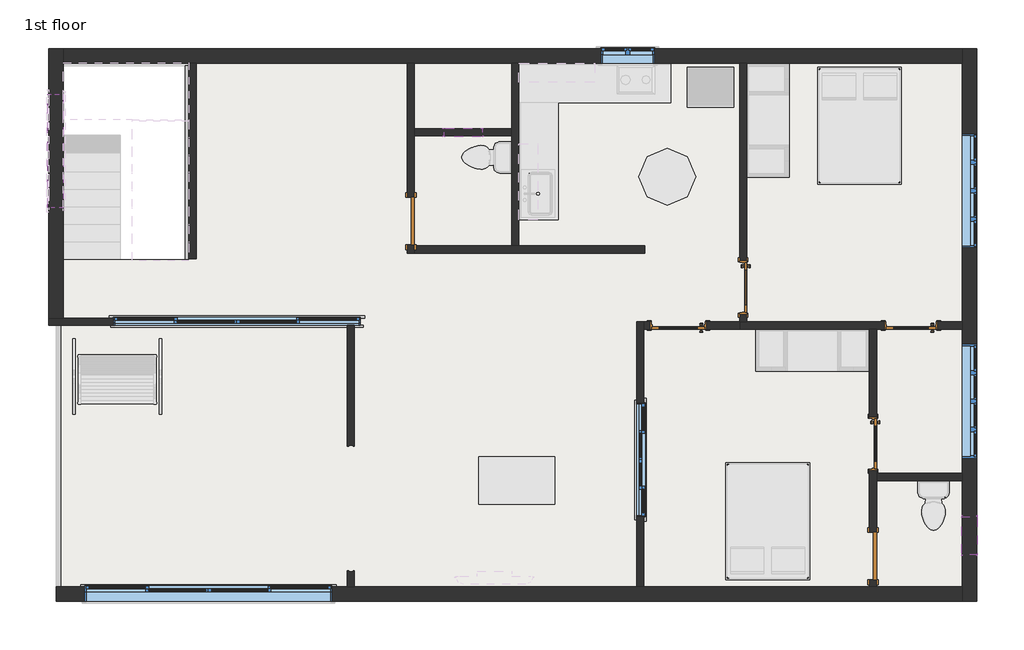
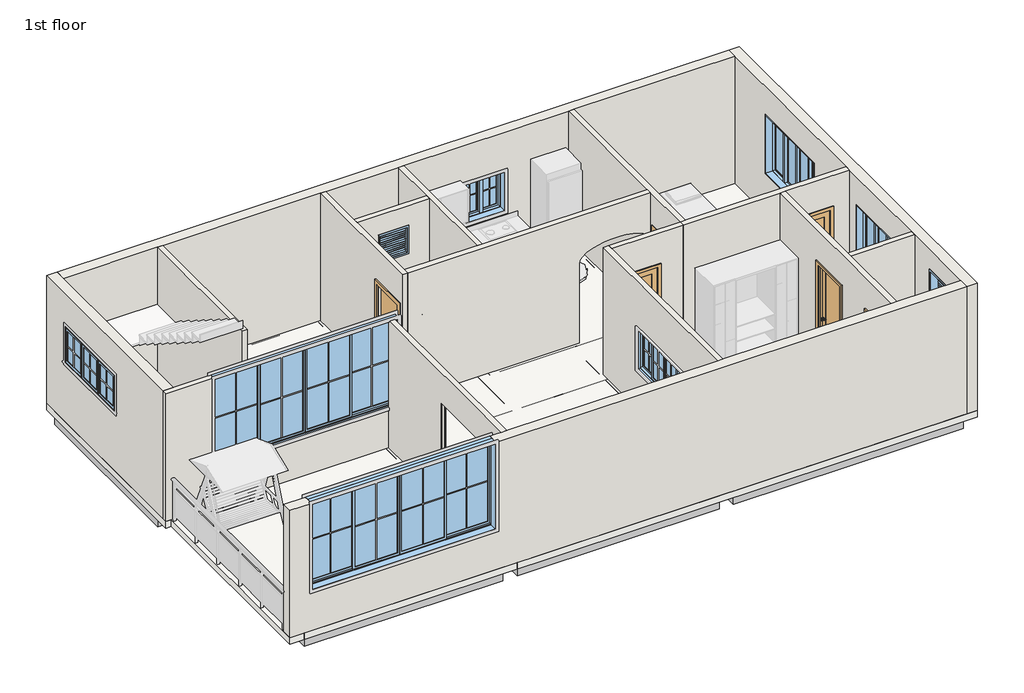
# One storey, part 1 of 2: 17 walls, 9 windows, 8 beams, 6 doors, 1 slab.
"""IFC4 building model written with IfcOpenShell, lengths in millimetres."""

from ifc_helpers import new_model, si_unit, point, frame, origin, place, context, project, spatial, polyline, ellipse_curve, trimmed, outline, extrude, faceted_brep, transform, mapped, element, save
from ifc_brep_helpers import plane_surface, extruded_surface, advanced_brep
from components import door_643e272e, door_51292941, door_214872d5, window_33d4544c, window_339605e1, window_5487fb6d, window_d39e7ecb, window_f2d8fef0, window_cbca41e3, window_8ea0b4a1, window_cd2bb1e7

model = new_model("IFC4")

# Units and contexts
model_context = context("Model", 3, world=origin())
ifc_project = project(units=[si_unit("LENGTHUNIT", "METRE", prefix="MILLI")], contexts=[model_context])

# Site, building, storey
site = spatial("IfcSite", under=ifc_project)
building = spatial("IfcBuilding", under=site)
storey = spatial("IfcBuildingStorey", under=building, Name="1st floor", Elevation=3810.0)

# Beams
placement = place(None, origin())
element("IfcBeam", 1, ObjectType="Concrete-Rectangular Beam", at=placement, inside=storey, context=model_context, shape_type="Brep", body=[
    faceted_brep([(-12452.868339, 913.093496, 3810.0), (-12452.868339, 684.493496, 3810.0), (-8179.318339, 684.493496, 3810.0), (-8179.318339, 913.093496, 3810.0), (-12452.868339, 913.093496, 3505.2), (-8179.318339, 913.093496, 3505.2), (-12452.868339, 684.493496, 3505.2), (-8179.318339, 684.493496, 3505.2)], [[[0, 1, 2, 3]], [[4, 0, 3, 5]], [[6, 4, 5, 7]], [[1, 6, 7, 2]], [[1, 0, 4, 6]], [[3, 2, 7, 5]]]),
    faceted_brep([(1713.981661, 913.093496, 3810.0), (1713.981661, 684.493496, 3810.0), (1713.981661, 684.493496, 3505.2), (1713.981661, 913.093496, 3505.2), (-3226.216739, 684.493496, 3810.0), (-3226.216739, 913.093496, 3810.0), (-3226.216739, 913.093496, 3505.2), (-3226.216739, 684.493496, 3505.2), (469.381661, 913.093496, 3810.0), (240.781661, 913.093496, 3810.0), (-1613.418339, 913.093496, 3810.0), (-1842.018339, 913.093496, 3810.0), (469.381661, 913.093496, 3505.2), (240.781661, 913.093496, 3505.2), (-1613.418339, 913.093496, 3505.2), (-1842.018339, 913.093496, 3505.2)], [[[0, 1, 2, 3]], [[4, 5, 6, 7]], [[1, 0, 8, 9, 10, 11, 5, 4]], [[0, 3, 12, 13, 14, 15, 6, 5, 11, 10, 9, 8]], [[3, 2, 7, 6, 15, 14, 13, 12]], [[2, 1, 4, 7]]]),
    faceted_brep([(-7874.518339, 684.493496, 3810.0), (-7874.518339, 913.093496, 3810.0), (-7874.518339, 913.093496, 3505.2), (-7874.518339, 684.493496, 3505.2), (-3531.016739, 684.493496, 3810.0), (-3531.016739, 913.093496, 3810.0), (-5271.018339, 913.093496, 3810.0), (-5499.618339, 913.093496, 3810.0), (-6947.418339, 913.093496, 3810.0), (-7176.018339, 913.093496, 3810.0), (-3531.016739, 913.093496, 3505.2), (-5271.018339, 913.093496, 3505.2), (-5499.618339, 913.093496, 3505.2), (-6947.418339, 913.093496, 3505.2), (-7176.018339, 913.093496, 3505.2), (-3531.016739, 684.493496, 3505.2)], [[[0, 1, 2, 3]], [[1, 0, 4, 5, 6, 7, 8, 9]], [[2, 1, 9, 8, 7, 6, 5, 10, 11, 12, 13, 14]], [[3, 2, 14, 13, 12, 11, 10, 15]], [[0, 3, 15, 4]], [[5, 4, 15, 10]]]),
])
element("IfcBeam", 2, ObjectType="Concrete-Rectangular Beam", at=placement, inside=storey, context=model_context, shape_type="SweptSolid", body=[
    extrude(outline(polyline([(-12871.968339, 9244.293496), (-12643.368339, 9244.293496), (-12643.368339, 5415.243496), (-12871.968339, 5415.243496), (-12871.968339, 9244.293496)])), frame((0.0, 0.0, 3505.2), z_axis=(0.0, 0.0, 1.0), x_axis=(1.0, 0.0, 0.0)), (0.0, 0.0, 1.0), 304.8),
])
element("IfcBeam", 3, ObjectType="Concrete-Rectangular Beam", at=placement, inside=storey, context=model_context, shape_type="Brep", body=[
    faceted_brep([(-10452.618339, 5110.443496, 3810.0), (-10681.218339, 5110.443496, 3810.0), (-10681.218339, 5110.443496, 3505.2), (-10452.618339, 5110.443496, 3505.2), (-10452.618339, 5148.543496, 3810.0), (-10452.618339, 5377.143496, 3810.0), (-10452.618339, 9282.393496, 3810.0), (-10681.218339, 9282.393496, 3810.0), (-10681.218339, 5377.143496, 3810.0), (-10681.218339, 5148.543496, 3810.0), (-10681.218339, 9282.393496, 3505.2), (-10681.218339, 5377.143496, 3505.2), (-10681.218339, 5148.543496, 3505.2), (-10452.618339, 9282.393496, 3505.2), (-10452.618339, 5377.143496, 3505.2), (-10452.618339, 5148.543496, 3505.2)], [[[0, 1, 2, 3]], [[1, 0, 4, 5, 6, 7, 8, 9]], [[2, 1, 9, 8, 7, 10, 11, 12]], [[3, 2, 12, 11, 10, 13, 14, 15]], [[0, 3, 15, 14, 13, 6, 5, 4]], [[7, 6, 13, 10]]]),
])
element("IfcBeam", 4, ObjectType="Concrete-Rectangular Beam", at=placement, inside=storey, context=model_context, shape_type="Brep", body=[
    faceted_brep([(-10452.618339, 5377.143496, 3810.0), (-10452.618339, 5148.543496, 3810.0), (-8274.568339, 5148.543496, 3810.0), (-8274.568339, 5339.043496, 3810.0), (-7969.768339, 5339.043496, 3810.0), (-7969.768339, 5148.543496, 3810.0), (-7912.618339, 5148.543496, 3810.0), (-7912.618339, 5224.743496, 3810.0), (-7912.618339, 5377.143496, 3810.0), (-7912.618339, 5148.543496, 3505.2), (-7969.768339, 5148.543496, 3505.2), (-10452.618339, 5148.543496, 3505.2), (-10452.618339, 5377.143496, 3505.2), (-7912.618339, 5377.143496, 3505.2), (-7912.618339, 5224.743496, 3505.2), (-7969.768339, 5339.043496, 3505.2), (-8274.568339, 5339.043496, 3505.2), (-8274.568339, 5148.543496, 3505.2)], [[[0, 1, 2, 3, 4, 5, 6, 7, 8]], [[9, 6, 5, 10]], [[11, 12, 13, 14, 9, 10, 15, 16, 17]], [[12, 0, 8, 13]], [[1, 0, 12, 11]], [[8, 7, 6, 9, 14, 13]], [[16, 3, 2, 17]], [[3, 16, 15, 4]], [[4, 15, 10, 5]], [[1, 11, 17, 2]]]),
    faceted_brep([(-12643.368339, 5148.543496, 3810.0), (-12643.368339, 5377.143496, 3810.0), (-12643.368339, 5377.143496, 3505.2), (-12643.368339, 5148.543496, 3505.2), (-10681.218339, 5377.143496, 3810.0), (-10681.218339, 5148.543496, 3810.0), (-10681.218339, 5148.543496, 3505.2), (-10681.218339, 5377.143496, 3505.2)], [[[0, 1, 2, 3]], [[4, 5, 6, 7]], [[1, 0, 5, 4]], [[3, 2, 7, 6]], [[2, 1, 4, 7]], [[0, 3, 6, 5]]]),
])
element("IfcBeam", 5, ObjectType="Concrete-Rectangular Beam", at=placement, inside=storey, context=model_context, shape_type="Brep", body=[
    faceted_brep([(-7912.618339, 5148.543496, 3810.0), (-7969.768339, 5148.543496, 3810.0), (-7969.768339, 5110.443496, 3810.0), (-8141.218339, 5110.443496, 3810.0), (-8141.218339, 913.093496, 3810.0), (-7912.618339, 913.093496, 3810.0), (-7912.618339, 4996.143496, 3810.0), (-7912.618339, 5148.543496, 3505.2), (-7912.618339, 913.093496, 3505.2), (-7912.618339, 4996.143496, 3505.2), (-7969.768339, 5148.543496, 3505.2), (-8141.218339, 913.093496, 3505.2), (-8141.218339, 5110.443496, 3505.2), (-7969.768339, 5110.443496, 3505.2)], [[[0, 1, 2, 3, 4, 5, 6]], [[7, 0, 6, 5, 8, 9]], [[10, 7, 9, 8, 11, 12, 13]], [[3, 12, 11, 4]], [[0, 7, 10, 1]], [[2, 13, 12, 3]], [[13, 2, 1, 10]], [[5, 4, 11, 8]]]),
])
element("IfcBeam", 6, ObjectType="Concrete-Rectangular Beam", at=placement, inside=storey, context=model_context, shape_type="Brep", body=[
    faceted_brep([(-6947.418339, 9282.393496, 3810.0), (-7176.018339, 9282.393496, 3810.0), (-7176.018339, 5224.743496, 3810.0), (-7176.018339, 4996.143496, 3810.0), (-7176.018339, 913.093496, 3810.0), (-6947.418339, 913.093496, 3810.0), (-6947.418339, 4996.143496, 3810.0), (-6947.418339, 5224.743496, 3810.0), (-6947.418339, 6215.343496, 3810.0), (-6947.418339, 6443.943496, 3810.0), (-6947.418339, 8094.943496, 3810.0), (-6947.418339, 8323.543496, 3810.0), (-7176.018339, 9282.393496, 3505.2), (-7176.018339, 5224.743496, 3505.2), (-7176.018339, 4996.143496, 3505.2), (-7176.018339, 913.093496, 3505.2), (-6947.418339, 9282.393496, 3505.2), (-6947.418339, 8323.543496, 3505.2), (-6947.418339, 8094.943496, 3505.2), (-6947.418339, 6443.943496, 3505.2), (-6947.418339, 6215.343496, 3505.2), (-6947.418339, 5224.743496, 3505.2), (-6947.418339, 4996.143496, 3505.2), (-6947.418339, 913.093496, 3505.2)], [[[0, 1, 2, 3, 4, 5, 6, 7, 8, 9, 10, 11]], [[1, 12, 13, 14, 15, 4, 3, 2]], [[12, 16, 17, 18, 19, 20, 21, 22, 23, 15, 14, 13]], [[16, 0, 11, 10, 9, 8, 7, 6, 5, 23, 22, 21, 20, 19, 18, 17]], [[1, 0, 16, 12]], [[5, 4, 15, 23]]]),
])
element("IfcBeam", 7, ObjectType="Concrete-Rectangular Beam", at=placement, inside=storey, context=model_context, shape_type="Brep", body=[
    faceted_brep([(-5271.018339, 9282.393496, 3810.0), (-5499.618339, 9282.393496, 3810.0), (-5499.618339, 8323.543496, 3810.0), (-5499.618339, 8094.943496, 3810.0), (-5499.618339, 6443.943496, 3810.0), (-5499.618339, 6215.343496, 3810.0), (-5499.618339, 5224.743496, 3810.0), (-5499.618339, 4996.143496, 3810.0), (-5499.618339, 913.093496, 3810.0), (-5271.018339, 913.093496, 3810.0), (-5271.018339, 4996.143496, 3810.0), (-5271.018339, 5224.743496, 3810.0), (-5271.018339, 6215.343496, 3810.0), (-5271.018339, 6443.943496, 3810.0), (-5499.618339, 9282.393496, 3505.2), (-5499.618339, 8323.543496, 3505.2), (-5499.618339, 8094.943496, 3505.2), (-5499.618339, 6443.943496, 3505.2), (-5499.618339, 6215.343496, 3505.2), (-5499.618339, 5224.743496, 3505.2), (-5499.618339, 4996.143496, 3505.2), (-5499.618339, 913.093496, 3505.2), (-5271.018339, 9282.393496, 3505.2), (-5271.018339, 6443.943496, 3505.2), (-5271.018339, 6215.343496, 3505.2), (-5271.018339, 5224.743496, 3505.2), (-5271.018339, 4996.143496, 3505.2), (-5271.018339, 913.093496, 3505.2)], [[[0, 1, 2, 3, 4, 5, 6, 7, 8, 9, 10, 11, 12, 13]], [[1, 14, 15, 16, 17, 18, 19, 20, 21, 8, 7, 6, 5, 4, 3, 2]], [[14, 22, 23, 24, 25, 26, 27, 21, 20, 19, 18, 17, 16, 15]], [[22, 0, 13, 12, 11, 10, 9, 27, 26, 25, 24, 23]], [[1, 0, 22, 14]], [[9, 8, 21, 27]]]),
])
element("IfcBeam", 8, ObjectType="Concrete-Rectangular Beam", at=placement, inside=storey, context=model_context, shape_type="Brep", body=[
    faceted_brep([(-7176.018339, 4996.143496, 3810.0), (-7176.018339, 5224.743496, 3810.0), (-7912.618339, 5224.743496, 3810.0), (-7912.618339, 5148.543496, 3810.0), (-7912.618339, 4996.143496, 3810.0), (-7176.018339, 5224.743496, 3505.2), (-7912.618339, 5224.743496, 3505.2), (-7176.018339, 4996.143496, 3505.2), (-7912.618339, 4996.143496, 3505.2), (-7912.618339, 5148.543496, 3505.2)], [[[0, 1, 2, 3, 4]], [[1, 5, 6, 2]], [[5, 7, 8, 9, 6]], [[4, 8, 7, 0]], [[1, 0, 7, 5]], [[8, 4, 3, 2, 6, 9]]]),
    faceted_brep([(-6947.418339, 4996.143496, 3810.0), (-6947.418339, 5224.743496, 3810.0), (-6947.418339, 5224.743496, 3505.2), (-6947.418339, 4996.143496, 3505.2), (-5499.618339, 4996.143496, 3810.0), (-5499.618339, 5224.743496, 3810.0), (-5499.618339, 5224.743496, 3505.2), (-5499.618339, 4996.143496, 3505.2)], [[[0, 1, 2, 3]], [[1, 0, 4, 5]], [[2, 1, 5, 6]], [[3, 2, 6, 7]], [[0, 3, 7, 4]], [[5, 4, 7, 6]]]),
    faceted_brep([(-5271.018339, 4996.143496, 3810.0), (-5271.018339, 5224.743496, 3810.0), (-5271.018339, 5224.743496, 3505.2), (-5271.018339, 4996.143496, 3505.2), (-3492.916739, 4996.143496, 3810.0), (-3264.316739, 4996.143496, 3810.0), (-1842.018339, 4996.143496, 3810.0), (-1842.018339, 5053.293496, 3810.0), (-2089.668339, 5053.293496, 3810.0), (-2089.668339, 5224.743496, 3810.0), (-3264.316739, 5224.743496, 3810.0), (-3492.916739, 5224.743496, 3810.0), (-2089.668339, 5224.743496, 3505.2), (-3264.316739, 5224.743496, 3505.2), (-3492.916739, 5224.743496, 3505.2), (-2089.668339, 5053.293496, 3505.2), (-1842.018339, 5053.293496, 3505.2), (-1842.018339, 4996.143496, 3505.2), (-3264.316739, 4996.143496, 3505.2), (-3492.916739, 4996.143496, 3505.2)], [[[0, 1, 2, 3]], [[1, 0, 4, 5, 6, 7, 8, 9, 10, 11]], [[2, 1, 11, 10, 9, 12, 13, 14]], [[3, 2, 14, 13, 12, 15, 16, 17, 18, 19]], [[0, 3, 19, 18, 17, 6, 5, 4]], [[6, 17, 16, 7]], [[15, 8, 7, 16]], [[8, 15, 12, 9]]]),
    faceted_brep([(-1613.418339, 4996.143496, 3810.0), (-1613.418339, 5224.743496, 3810.0), (-1613.418339, 5224.743496, 3505.2), (-1613.418339, 4996.143496, 3505.2), (240.781661, 4996.143496, 3810.0), (469.381661, 4996.143496, 3810.0), (1790.181661, 4996.143496, 3810.0), (1790.181661, 5224.743496, 3810.0), (1790.181661, 5224.743496, 3505.2), (1790.181661, 4996.143496, 3505.2), (469.381661, 4996.143496, 3505.2), (240.781661, 4996.143496, 3505.2)], [[[0, 1, 2, 3]], [[1, 0, 4, 5, 6, 7]], [[3, 2, 8, 9, 10, 11]], [[0, 3, 11, 10, 9, 6, 5, 4]], [[2, 1, 7, 8]], [[7, 6, 9, 8]]]),
])

# Doors
door_shape = door_643e272e(model_context)
element("IfcDoor", 9, ObjectType="Door-Interior-Single-1_Panel-Wood : 32\" x 84\"", at=placement, inside=storey, context=model_context, shape_type="MappedRepresentation", body=[
    mapped(door_shape, transform((-1724.543339, 5720.043496, 3810.0), x_axis=(0.0, -1.0, 0.0), y_axis=(1.0, 0.0, 0.0), z_axis=(0.0, 0.0, 1.0))),
])
element("IfcDoor", 10, ObjectType="Door-Interior-Single-1_Panel-Wood : 32\" x 84\"", at=placement, inside=storey, context=model_context, shape_type="MappedRepresentation", body=[
    mapped(door_shape, transform((358.256661, 3211.793496, 3810.0), x_axis=(0.0, -1.0, 0.0), y_axis=(1.0, 0.0, 0.0), z_axis=(0.0, 0.0, 1.0))),
])
element("IfcDoor", 11, ObjectType="Door-Interior-Single-1_Panel-Wood : 32\" x 84\"", at=placement, inside=storey, context=model_context, shape_type="MappedRepresentation", body=[
    mapped(door_shape, transform((964.681661, 5107.268496, 3810.0), x_axis=(-1.0, 0.0, 0.0), y_axis=(0.0, -1.0, 0.0), z_axis=(0.0, 0.0, 1.0))),
])
door_2_shape = door_51292941(model_context)
element("IfcDoor", 12, ObjectType="Door-Interior-Single-1_Panel-Wood : 34\" x 84\"", at=placement, inside=storey, context=model_context, shape_type="MappedRepresentation", body=[
    mapped(door_2_shape, transform((-2769.016739, 5107.268496, 3810.0), x_axis=(-1.0, 0.0, 0.0), y_axis=(0.0, -1.0, 0.0), z_axis=(0.0, 0.0, 1.0))),
])
door_3_shape = door_214872d5(model_context)
element("IfcDoor", 13, ObjectType="Single-Flush : 30\" x 84\"", at=placement, inside=storey, context=model_context, shape_type="MappedRepresentation", body=[
    mapped(door_3_shape, transform((355.081661, 1408.393496, 3810.0), x_axis=(0.0, -1.0, 0.0), y_axis=(1.0, 0.0, 0.0), z_axis=(0.0, 0.0, 1.0))),
])
element("IfcDoor", 14, ObjectType="Single-Flush : 30\" x 84\"", at=placement, inside=storey, context=model_context, shape_type="MappedRepresentation", body=[
    mapped(door_3_shape, transform((-7061.718339, 6786.843496, 3810.0), x_axis=(0.0, -1.0, 0.0), y_axis=(1.0, 0.0, 0.0), z_axis=(0.0, 0.0, 1.0))),
])

# Slab
element("IfcSlab", 15, ObjectType="Generic - 6\"", at=placement, inside=storey, context=model_context, shape_type="SweptSolid", body=[
    extrude(outline(polyline([(2018.781661, 9549.093496), (2018.781661, 684.493496), (-12757.668339, 684.493496), (-12757.668339, 5110.443496), (-12871.968339, 5110.443496), (-12871.968339, 9549.093496), (2018.781661, 9549.093496)]), holes=[polyline([(-10624.068339, 9320.493496), (-12643.368339, 9320.493496), (-12643.368339, 6177.243496), (-10624.068339, 6177.243496), (-10624.068339, 9320.493496)])]), frame((0.0, 0.0, 3657.6), z_axis=(0.0, 0.0, 1.0), x_axis=(1.0, 0.0, 0.0)), (0.0, 0.0, 1.0), 152.4),
])

# Walls
element("IfcWall", 16, ObjectType="Generic - 4.5\"", at=placement, inside=storey, context=model_context, shape_type="SweptSolid", body=[
    extrude(outline(polyline([(-10624.068339, 6177.243496), (-10624.068339, 9320.493496), (-10509.768339, 9320.493496), (-10509.768339, 6177.243496), (-10624.068339, 6177.243496)])), frame((0.0, 0.0, 3810.0), z_axis=(0.0, 0.0, 1.0), x_axis=(1.0, 0.0, 0.0)), (0.0, 0.0, 1.0), 2895.6),
])
element("IfcWall", 17, ObjectType="Generic - 4.5\"", at=placement, inside=storey, context=model_context, shape_type="Brep", body=[
    faceted_brep([(-7118.868339, 6405.843496, 5943.6), (-7118.868339, 6405.843496, 3810.0), (-7118.868339, 6272.493496, 3810.0), (-7118.868339, 6272.493496, 6705.6), (-7118.868339, 9320.493496, 6705.6), (-7118.868339, 9320.493496, 3810.0), (-7118.868339, 7167.843496, 3810.0), (-7118.868339, 7167.843496, 5943.6), (-7004.568339, 6272.493496, 3810.0), (-7004.568339, 6386.793496, 3810.0), (-7004.568339, 6405.843496, 3810.0), (-7004.568339, 6405.843496, 5943.6), (-7004.568339, 7167.843496, 5943.6), (-7004.568339, 7167.843496, 3810.0), (-7004.568339, 8152.093496, 3810.0), (-7004.568339, 8266.393496, 3810.0), (-7004.568339, 9320.493496, 3810.0), (-7004.568339, 9320.493496, 6705.6), (-7004.568339, 8266.393496, 6705.6), (-7004.568339, 8152.093496, 6705.6), (-7004.568339, 6386.793496, 6705.6), (-7004.568339, 6272.493496, 6705.6)], [[[0, 1, 2, 3, 4, 5, 6, 7]], [[8, 9, 10, 11, 12, 13, 14, 15, 16, 17, 18, 19, 20, 21]], [[6, 5, 16, 15, 14, 13]], [[2, 1, 10, 9, 8]], [[4, 3, 21, 20, 19, 18, 17]], [[3, 2, 8, 21]], [[5, 4, 17, 16]], [[11, 10, 1, 0]], [[12, 11, 0, 7]], [[13, 12, 7, 6]]]),
])
element("IfcWall", 18, ObjectType="Generic - 4.5\"", at=placement, inside=storey, context=model_context, shape_type="Brep", body=[
    faceted_brep([(-5442.468339, 9320.493496, 3810.0), (-5442.468339, 8266.393496, 3810.0), (-5442.468339, 8152.093496, 3810.0), (-5442.468339, 6386.793496, 3810.0), (-5442.468339, 6386.793496, 6705.6), (-5442.468339, 8152.093496, 6705.6), (-5442.468339, 8266.393496, 6705.6), (-5442.468339, 9320.493496, 6705.6), (-5328.168339, 9320.493496, 3810.0), (-5328.168339, 9320.493496, 6705.6), (-5328.168339, 6386.793496, 6705.6), (-5328.168339, 6386.793496, 3810.0)], [[[0, 1, 2, 3, 4, 5, 6, 7]], [[8, 9, 10, 11]], [[3, 2, 1, 0, 8, 11]], [[7, 6, 5, 4, 10, 9]], [[4, 3, 11, 10]], [[0, 7, 9, 8]]]),
])
element("IfcWall", 19, ObjectType="Generic - 4.5\"", at=placement, inside=storey, context=model_context, shape_type="Brep", body=[
    faceted_brep([(-1784.868339, 5167.593496, 6705.6), (-1784.868339, 6272.493496, 6705.6), (-1784.868339, 6386.793496, 6705.6), (-1784.868339, 9320.493496, 6705.6), (-1784.868339, 9320.493496, 3810.0), (-1784.868339, 6386.793496, 3810.0), (-1784.868339, 6272.493496, 3810.0), (-1784.868339, 6151.843496, 3810.0), (-1784.868339, 6151.843496, 5969.0), (-1784.868339, 5288.243496, 5969.0), (-1784.868339, 5288.243496, 3810.0), (-1784.868339, 5167.593496, 3810.0), (-1670.568339, 9320.493496, 6705.6), (-1670.568339, 5167.593496, 6705.6), (-1670.568339, 5167.593496, 3810.0), (-1670.568339, 5288.243496, 3810.0), (-1670.568339, 5288.243496, 5969.0), (-1670.568339, 6151.843496, 5969.0), (-1670.568339, 6151.843496, 3810.0), (-1670.568339, 9320.493496, 3810.0)], [[[0, 1, 2, 3, 4, 5, 6, 7, 8, 9, 10, 11]], [[12, 13, 14, 15, 16, 17, 18, 19]], [[14, 11, 10, 15]], [[4, 19, 18, 7, 6, 5]], [[3, 2, 1, 0, 13, 12]], [[0, 11, 14, 13]], [[4, 3, 12, 19]], [[9, 16, 15, 10]], [[16, 9, 8, 17]], [[17, 8, 7, 18]]]),
])
element("IfcWall", 20, ObjectType="Generic - 4.5\"", at=placement, inside=storey, context=model_context, shape_type="Brep", body=[
    faceted_brep([(-1784.868339, 5167.593496, 6705.6), (-1670.568339, 5167.593496, 6705.6), (1790.181661, 5167.593496, 6705.6), (1790.181661, 5167.593496, 3810.0), (1396.481661, 5167.593496, 3810.0), (1396.481661, 5167.593496, 5969.0), (532.881661, 5167.593496, 5969.0), (532.881661, 5167.593496, 3810.0), (-1670.568339, 5167.593496, 3810.0), (-1784.868339, 5167.593496, 3810.0), (1790.181661, 5053.293496, 6705.6), (412.231661, 5053.293496, 6705.6), (297.931661, 5053.293496, 6705.6), (-1784.868339, 5053.293496, 6705.6), (-1784.868339, 5053.293496, 3810.0), (297.931661, 5053.293496, 3810.0), (412.231661, 5053.293496, 3810.0), (532.881661, 5053.293496, 3810.0), (532.881661, 5053.293496, 5969.0), (1396.481661, 5053.293496, 5969.0), (1396.481661, 5053.293496, 3810.0), (1790.181661, 5053.293496, 3810.0)], [[[0, 1, 2, 3, 4, 5, 6, 7, 8, 9]], [[10, 11, 12, 13, 14, 15, 16, 17, 18, 19, 20, 21]], [[3, 21, 20, 4]], [[14, 9, 8, 7, 17, 16, 15]], [[2, 1, 0, 13, 12, 11, 10]], [[3, 2, 10, 21]], [[0, 9, 14, 13]], [[6, 18, 17, 7]], [[18, 6, 5, 19]], [[19, 5, 4, 20]]]),
])
element("IfcWall", 21, ObjectType="Generic - 4.5\"", at=placement, inside=storey, context=model_context, shape_type="AdvancedBrep", body=[
    advanced_brep(
    [(-1784.868339, 6272.493496, 6705.6), (-7004.568339, 6272.493496, 6705.6), (-7004.568339, 6272.493496, 3810.0), (-3308.868339, 6272.493496, 3810.0), (-3308.868339, 6272.493496, 5638.8), (-1784.868339, 6272.493496, 5638.8), (-7004.568339, 6386.793496, 6705.6), (-5442.468339, 6386.793496, 6705.6), (-5328.168339, 6386.793496, 6705.6), (-1784.868339, 6386.793496, 6705.6), (-1784.868339, 6386.793496, 5638.8), (-3308.868339, 6386.793496, 5638.8), (-3308.868339, 6386.793496, 3810.0), (-5328.168339, 6386.793496, 3810.0), (-5442.468339, 6386.793496, 3810.0), (-7004.568339, 6386.793496, 3810.0)],
    [
        (0, 1),
        (1, 2),
        (2, 3),
        (3, 4),
        (4, 5, ellipse_curve(frame((-2546.868339, 6272.493496, 5638.8), z_axis=(0.0, 1.0, 0.0), x_axis=(1.0, 0.0, 0.0)), 762.0, 304.8)),
        (5, 0),
        (6, 7),
        (7, 8),
        (8, 9),
        (9, 10),
        (10, 11, ellipse_curve(frame((-2546.868339, 6386.793496, 5638.8), z_axis=(0.0, -1.0, 0.0), x_axis=(1.0, 0.0, 0.0)), 762.0, 304.8)),
        (11, 12),
        (12, 13),
        (13, 14),
        (14, 15),
        (15, 6),
        (2, 15),
        (12, 3),
        (0, 9),
        (6, 1),
        (5, 10),
        (4, 11),
    ],
    [
        plane_surface(frame((-7061.718339, 6272.493496, 3810.0), z_axis=(0.0, -1.0, 0.0), x_axis=(1.0, 0.0, 0.0))),
        plane_surface(frame((-7061.718339, 6386.793496, 3810.0), z_axis=(0.0, 1.0, 0.0), x_axis=(-1.0, 0.0, 0.0))),
        plane_surface(frame((-7061.718339, 6272.493496, 3810.0), z_axis=(0.0, 0.0, -1.0), x_axis=(0.0, 1.0, 0.0))),
        plane_surface(frame((-1727.718339, 6272.493496, 6705.6), z_axis=(0.0, 0.0, 1.0), x_axis=(0.0, 1.0, 0.0))),
        plane_surface(frame((-7004.568339, 9377.643496, 3810.0), z_axis=(-1.0, 0.0, 0.0), x_axis=(0.0, 1.0, 0.0))),
        plane_surface(frame((-1784.868339, 9377.643496, 3810.0), z_axis=(1.0, 0.0, 0.0), x_axis=(0.0, -1.0, 0.0))),
        extruded_surface(trimmed(ellipse_curve(frame((-2546.868339, 7796.493496, 5638.8), z_axis=(0.0, -1.0, 0.0), x_axis=(1.0, 0.0, 0.0)), 762.0, 304.8), [point((-1784.868339, 7796.493496, 5638.8))], [point((-3308.868339, 7796.493496, 5638.8))], True, "CARTESIAN"), (0.0, 3047.999999999999, 0.0), 3047.999999999999),
        plane_surface(frame((-3308.868339, 4748.493496, 5638.8), z_axis=(1.0, 0.0, 0.0), x_axis=(0.0, 1.0, 0.0))),
    ],
    [
        (0, [[1, 2, 3, 4, 5, 6]]),
        (1, [[7, 8, 9, 10, 11, 12, 13, 14, 15, 16]]),
        (2, [[17, -15, -14, -13, 18, -3]]),
        (3, [[-1, 19, -9, -8, -7, 20]]),
        (4, [[-2, -20, -16, -17]]),
        (5, [[-19, -6, 21, -10]]),
        (6, [[22, -11, -21, -5]]),
        (7, [[-22, -4, -18, -12]]),
    ],
),
])
element("IfcWall", 22, ObjectType="Generic - 4.5\"", at=placement, inside=storey, context=model_context, shape_type="Brep", body=[
    faceted_brep([(297.931661, 913.093496, 6705.6), (297.931661, 5053.293496, 6705.6), (297.931661, 5053.293496, 3810.0), (297.931661, 3643.593496, 3810.0), (297.931661, 3643.593496, 5969.0), (297.931661, 2779.993496, 5969.0), (297.931661, 2779.993496, 3810.0), (297.931661, 1789.393496, 3810.0), (297.931661, 1789.393496, 5943.6), (297.931661, 1027.393496, 5943.6), (297.931661, 1027.393496, 3810.0), (297.931661, 913.093496, 3810.0), (412.231661, 5053.293496, 6705.6), (412.231661, 2735.543496, 6705.6), (412.231661, 2621.243496, 6705.6), (412.231661, 913.093496, 6705.6), (412.231661, 913.093496, 3810.0), (412.231661, 1027.393496, 3810.0), (412.231661, 1027.393496, 5943.6), (412.231661, 1789.393496, 5943.6), (412.231661, 1789.393496, 3810.0), (412.231661, 2621.243496, 3810.0), (412.231661, 2735.543496, 3810.0), (412.231661, 2779.993496, 3810.0), (412.231661, 2779.993496, 5969.0), (412.231661, 3643.593496, 5969.0), (412.231661, 3643.593496, 3810.0), (412.231661, 5053.293496, 3810.0)], [[[0, 1, 2, 3, 4, 5, 6, 7, 8, 9, 10, 11]], [[12, 13, 14, 15, 16, 17, 18, 19, 20, 21, 22, 23, 24, 25, 26, 27]], [[2, 27, 26, 3]], [[16, 11, 10, 17]], [[20, 7, 6, 23, 22, 21]], [[1, 0, 15, 14, 13, 12]], [[2, 1, 12, 27]], [[0, 11, 16, 15]], [[18, 17, 10, 9]], [[19, 18, 9, 8]], [[20, 19, 8, 7]], [[5, 24, 23, 6]], [[24, 5, 4, 25]], [[25, 4, 3, 26]]]),
])
element("IfcWall", 23, ObjectType="Generic - 4.5\"", at=placement, inside=storey, context=model_context, shape_type="SweptSolid", body=[
    extrude(outline(polyline([(1790.181661, 2621.243496), (412.231661, 2621.243496), (412.231661, 2735.543496), (1790.181661, 2735.543496), (1790.181661, 2621.243496)])), frame((0.0, 0.0, 3810.0), z_axis=(0.0, 0.0, 1.0), x_axis=(1.0, 0.0, 0.0)), (0.0, 0.0, 1.0), 2895.6),
])
element("IfcWall", 24, ObjectType="Generic - 4.5\"", at=placement, inside=storey, context=model_context, shape_type="Brep", body=[
    faceted_brep([(-3435.766739, 5167.593496, 3810.0), (-3435.766739, 913.093496, 3810.0), (-3435.766739, 913.093496, 6705.6), (-3435.766739, 5167.593496, 6705.6), (-3435.766739, 2040.218496, 5638.8), (-3435.766739, 2040.218496, 4724.4), (-3435.766739, 3869.018496, 4724.4), (-3435.766739, 3869.018496, 5638.8), (-3321.466739, 5167.593496, 3810.0), (-3321.466739, 5167.593496, 6705.6), (-3321.466739, 5053.293496, 6705.6), (-3321.466739, 913.093496, 6705.6), (-3321.466739, 913.093496, 3810.0), (-3321.466739, 5053.293496, 3810.0), (-3321.466739, 2040.218496, 5638.8), (-3321.466739, 3869.018496, 5638.8), (-3321.466739, 3869.018496, 4724.4), (-3321.466739, 2040.218496, 4724.4)], [[[0, 1, 2, 3], [4, 5, 6, 7]], [[8, 9, 10, 11, 12, 13], [14, 15, 16, 17]], [[1, 0, 8, 13, 12]], [[3, 2, 11, 10, 9]], [[2, 1, 12, 11]], [[0, 3, 9, 8]], [[5, 4, 14, 17]], [[6, 5, 17, 16]], [[7, 6, 16, 15]], [[4, 7, 15, 14]]]),
])
element("IfcWall", 25, ObjectType="Generic - 4.5\"", at=placement, inside=storey, context=model_context, shape_type="Brep", body=[
    faceted_brep([(-8084.068339, 913.093496, 3810.0), (-8084.068339, 913.093496, 6705.6), (-8084.068339, 5110.443496, 6705.6), (-8084.068339, 5110.443496, 4724.4), (-8084.068339, 5224.743496, 4724.4), (-8084.068339, 5224.743496, 3810.0), (-8084.068339, 5110.443496, 3810.0), (-8084.068339, 3170.393496, 3810.0), (-8084.068339, 3170.393496, 6019.0), (-8084.068339, 1170.393496, 6019.0), (-8084.068339, 1170.393496, 3810.0), (-7969.768339, 913.093496, 6705.6), (-7969.768339, 913.093496, 3810.0), (-7969.768339, 1170.393496, 3810.0), (-7969.768339, 1170.393496, 6019.0), (-7969.768339, 3170.393496, 6019.0), (-7969.768339, 3170.393496, 3810.0), (-7969.768339, 5224.743496, 3810.0), (-7969.768339, 5224.743496, 4724.4), (-7969.768339, 5110.443496, 4724.4), (-7969.768339, 5110.443496, 6705.6), (-8059.7683389, 1170.393496, 3810.0), (-8059.7683389, 1155.393496, 3810.0), (-7989.7683389, 1155.393496, 3810.0), (-7989.7683389, 1170.393496, 3810.0), (-7989.7683389, 3170.393496, 3810.0), (-7989.7683389, 3185.393496, 3810.0), (-8059.7683389, 3185.393496, 3810.0), (-8059.7683389, 3170.393496, 3810.0), (-7989.7683389, 1170.393496, 6019.0), (-7989.7683389, 3170.393496, 6019.0), (-8059.7683389, 3170.393496, 6019.0), (-8059.7683389, 1170.393496, 6019.0), (-8059.7683389, 3185.393496, 6034.0), (-8059.7683389, 1155.393496, 6034.0), (-7989.7683389, 1155.393496, 6034.0), (-7989.7683389, 3185.393496, 6034.0)], [[[0, 1, 2, 3, 4, 5, 6, 7, 8, 9, 10]], [[11, 12, 13, 14, 15, 16, 17, 18, 19, 20]], [[12, 0, 10, 21, 22, 23, 24, 13]], [[5, 17, 16, 25, 26, 27, 28, 7, 6]], [[1, 11, 20, 2]], [[1, 0, 12, 11]], [[17, 5, 4, 18]], [[29, 30, 15, 14]], [[31, 32, 9, 8]], [[28, 31, 8, 7]], [[32, 21, 10, 9]], [[32, 31, 28, 27, 33, 34, 22, 21]], [[22, 34, 35, 23]], [[30, 29, 24, 23, 35, 36, 26, 25]], [[24, 29, 14, 13]], [[30, 25, 16, 15]], [[33, 27, 26, 36]], [[34, 33, 36, 35]], [[19, 3, 2, 20]], [[3, 19, 18, 4]]]),
])
element("IfcWall", 26, ObjectType="Generic - 4.5\"", at=placement, inside=storey, context=model_context, shape_type="Brep", body=[
    faceted_brep([(-8084.068339, 5224.743496, 3810.0), (-12643.368339, 5224.743496, 3810.0), (-12871.968339, 5224.743496, 3810.0), (-12871.968339, 5224.743496, 6705.6), (-12643.368339, 5224.743496, 6705.6), (-11836.918339, 5224.743496, 6705.6), (-11836.918339, 5224.743496, 4724.4), (-8084.068339, 5224.743496, 4724.4), (-12871.968339, 5110.443496, 3810.0), (-8084.068339, 5110.443496, 3810.0), (-8084.068339, 5110.443496, 4724.4), (-11836.918339, 5110.443496, 4724.4), (-11836.918339, 5110.443496, 6705.6), (-12871.968339, 5110.443496, 6705.6)], [[[0, 1, 2, 3, 4, 5, 6, 7]], [[8, 9, 10, 11, 12, 13]], [[2, 1, 0, 9, 8]], [[3, 13, 12, 5, 4]], [[9, 0, 7, 10]], [[3, 2, 8, 13]], [[6, 11, 10, 7]], [[11, 6, 5, 12]]]),
])
element("IfcWall", 27, ObjectType="Generic - 4.5\"", at=placement, inside=storey, context=model_context, shape_type="SweptSolid", body=[
    extrude(outline(polyline([(6705.6, -1784.868339), (6705.6, -3321.466739), (3810.0, -3321.466739), (3810.0, -3226.216739), (5969.0, -3226.216739), (5969.0, -2311.816739), (3810.0, -2311.816739), (3810.0, -1784.868339), (6705.6, -1784.868339)])), frame((0.0, 5053.293496, 0.0), z_axis=(0.0, 1.0, 0.0), x_axis=(0.0, 0.0, 1.0)), (0.0, 0.0, 1.0), 114.3),
])
element("IfcWall", 28, ObjectType="Generic - 4.5\"", at=placement, inside=storey, context=model_context, shape_type="SweptSolid", body=[
    extrude(outline(polyline([(3810.0, -7004.568339), (3810.0, -5442.468339), (6705.6, -5442.468339), (6705.6, -7004.568339), (3810.0, -7004.568339)]), holes=[polyline([(6248.4, -6528.318339), (6248.4, -5918.718339), (5638.8, -5918.718339), (5638.8, -6528.318339), (6248.4, -6528.318339)])]), frame((0.0, 8152.093496, 0.0), z_axis=(0.0, 1.0, 0.0), x_axis=(0.0, 0.0, 1.0)), (0.0, 0.0, 1.0), 114.3),
])
element("IfcWall", 29, ObjectType="Generic - 9\"", at=placement, inside=storey, context=model_context, shape_type="Brep", body=[
    faceted_brep([(1790.181661, 9549.093496, 3810.0), (1790.181661, 9320.493496, 3810.0), (1790.181661, 5167.593496, 3810.0), (1790.181661, 5053.293496, 3810.0), (1790.181661, 2735.543496, 3810.0), (1790.181661, 2621.243496, 3810.0), (1790.181661, 913.093496, 3810.0), (1790.181661, 684.493496, 3810.0), (1790.181661, 684.493496, 6705.6), (1790.181661, 913.093496, 6705.6), (1790.181661, 2621.243496, 6705.6), (1790.181661, 2735.543496, 6705.6), (1790.181661, 5053.293496, 6705.6), (1790.181661, 5167.593496, 6705.6), (1790.181661, 9320.493496, 6705.6), (1790.181661, 9549.093496, 6705.6), (1790.181661, 6358.218496, 6070.6), (1790.181661, 6358.218496, 4724.4), (1790.181661, 8187.018496, 4724.4), (1790.181661, 8187.018496, 6070.6), (1790.181661, 2043.393496, 6248.4), (1790.181661, 1433.793496, 6248.4), (1790.181661, 1433.793496, 5638.8), (1790.181661, 2043.393496, 5638.8), (1790.181661, 2980.018496, 6070.6), (1790.181661, 2980.018496, 4724.4), (1790.181661, 4808.818496, 4724.4), (1790.181661, 4808.818496, 6070.6), (2018.781661, 9549.093496, 3810.0), (2018.781661, 9549.093496, 6705.6), (2018.781661, 684.493496, 6705.6), (2018.781661, 684.493496, 3810.0), (2018.781661, 6358.218496, 6070.6), (2018.781661, 8187.018496, 6070.6), (2018.781661, 8187.018496, 4724.4), (2018.781661, 6358.218496, 4724.4), (2018.781661, 2043.393496, 6248.4), (2018.781661, 2043.393496, 5638.8), (2018.781661, 1433.793496, 5638.8), (2018.781661, 1433.793496, 6248.4), (2018.781661, 2980.018496, 6070.6), (2018.781661, 4808.818496, 6070.6), (2018.781661, 4808.818496, 4724.4), (2018.781661, 2980.018496, 4724.4)], [[[0, 1, 2, 3, 4, 5, 6, 7, 8, 9, 10, 11, 12, 13, 14, 15], [16, 17, 18, 19], [20, 21, 22, 23], [24, 25, 26, 27]], [[28, 29, 30, 31], [32, 33, 34, 35], [36, 37, 38, 39], [40, 41, 42, 43]], [[7, 6, 5, 4, 3, 2, 1, 0, 28, 31]], [[15, 14, 13, 12, 11, 10, 9, 8, 30, 29]], [[0, 15, 29, 28]], [[8, 7, 31, 30]], [[17, 16, 32, 35]], [[18, 17, 35, 34]], [[19, 18, 34, 33]], [[16, 19, 33, 32]], [[37, 36, 20, 23]], [[38, 37, 23, 22]], [[39, 38, 22, 21]], [[36, 39, 21, 20]], [[25, 24, 40, 43]], [[26, 25, 43, 42]], [[27, 26, 42, 41]], [[24, 27, 41, 40]]]),
])
element("IfcWall", 30, ObjectType="Generic - 9\"", at=placement, inside=storey, context=model_context, shape_type="Brep", body=[
    faceted_brep([(1790.181661, 913.093496, 3810.0), (412.231661, 913.093496, 3810.0), (297.931661, 913.093496, 3810.0), (-3321.466739, 913.093496, 3810.0), (-3435.766739, 913.093496, 3810.0), (-7969.768339, 913.093496, 3810.0), (-8084.068339, 913.093496, 3810.0), (-12757.668339, 913.093496, 3810.0), (-12757.668339, 913.093496, 6705.6), (-12294.118339, 913.093496, 6705.6), (-12294.118339, 913.093496, 4724.4), (-8331.718339, 913.093496, 4724.4), (-8331.718339, 913.093496, 6705.6), (-8084.068339, 913.093496, 6705.6), (-7969.768339, 913.093496, 6705.6), (-3435.766739, 913.093496, 6705.6), (-3321.466739, 913.093496, 6705.6), (297.931661, 913.093496, 6705.6), (412.231661, 913.093496, 6705.6), (1790.181661, 913.093496, 6705.6), (-12757.668339, 684.493496, 3810.0), (1790.181661, 684.493496, 3810.0), (1790.181661, 684.493496, 6705.6), (-8331.718339, 684.493496, 6705.6), (-8331.718339, 684.493496, 4724.4), (-12294.118339, 684.493496, 4724.4), (-12294.118339, 684.493496, 6705.6), (-12757.668339, 684.493496, 6705.6)], [[[0, 1, 2, 3, 4, 5, 6, 7, 8, 9, 10, 11, 12, 13, 14, 15, 16, 17, 18, 19]], [[20, 21, 22, 23, 24, 25, 26, 27]], [[7, 6, 5, 4, 3, 2, 1, 0, 21, 20]], [[8, 7, 20, 27]], [[8, 27, 26, 9]], [[22, 19, 18, 17, 16, 15, 14, 13, 12, 23]], [[0, 19, 22, 21]], [[11, 24, 23, 12]], [[24, 11, 10, 25]], [[25, 10, 9, 26]]]),
])
element("IfcWall", 31, ObjectType="Generic - 9\"", at=placement, inside=storey, context=model_context, shape_type="Brep", body=[
    faceted_brep([(-12871.968339, 9549.093496, 3810.0), (-12871.968339, 5224.743496, 3810.0), (-12871.968339, 5224.743496, 6705.6), (-12871.968339, 9549.093496, 6705.6), (-12871.968339, 6996.393496, 5994.4), (-12871.968339, 6996.393496, 5181.6), (-12871.968339, 8825.193496, 5181.6), (-12871.968339, 8825.193496, 5994.4), (-12643.368339, 9549.093496, 3810.0), (-12643.368339, 9549.093496, 6705.6), (-12643.368339, 9320.493496, 6705.6), (-12643.368339, 5224.743496, 6705.6), (-12643.368339, 5224.743496, 3810.0), (-12643.368339, 9320.493496, 3810.0), (-12643.368339, 6996.393496, 5994.4), (-12643.368339, 8825.193496, 5994.4), (-12643.368339, 8825.193496, 5181.6), (-12643.368339, 6996.393496, 5181.6)], [[[0, 1, 2, 3], [4, 5, 6, 7]], [[8, 9, 10, 11, 12, 13], [14, 15, 16, 17]], [[1, 0, 8, 13, 12]], [[3, 2, 11, 10, 9]], [[0, 3, 9, 8]], [[2, 1, 12, 11]], [[5, 4, 14, 17]], [[6, 5, 17, 16]], [[7, 6, 16, 15]], [[4, 7, 15, 14]]]),
])
element("IfcWall", 32, ObjectType="Generic - 9\"", at=placement, inside=storey, context=model_context, shape_type="Brep", body=[
    faceted_brep([(-12643.368339, 9320.493496, 3810.0), (-10624.068339, 9320.493496, 3810.0), (-10509.768339, 9320.493496, 3810.0), (-7118.868339, 9320.493496, 3810.0), (-7004.568339, 9320.493496, 3810.0), (-5442.468339, 9320.493496, 3810.0), (-5328.168339, 9320.493496, 3810.0), (-1784.868339, 9320.493496, 3810.0), (-1670.568339, 9320.493496, 3810.0), (1790.181661, 9320.493496, 3810.0), (1790.181661, 9320.493496, 6705.6), (-1670.568339, 9320.493496, 6705.6), (-1784.868339, 9320.493496, 6705.6), (-5328.168339, 9320.493496, 6705.6), (-5442.468339, 9320.493496, 6705.6), (-7004.568339, 9320.493496, 6705.6), (-7118.868339, 9320.493496, 6705.6), (-10509.768339, 9320.493496, 6705.6), (-10624.068339, 9320.493496, 6705.6), (-12643.368339, 9320.493496, 6705.6), (-3150.118339, 9320.493496, 5829.3), (-3150.118339, 9320.493496, 4914.9), (-4013.718339, 9320.493496, 4914.9), (-4013.718339, 9320.493496, 5829.3), (-12643.368339, 9549.093496, 3810.0), (-12643.368339, 9549.093496, 6705.6), (1790.181661, 9549.093496, 6705.6), (1790.181661, 9549.093496, 3810.0), (-3150.118339, 9549.093496, 5829.3), (-4013.718339, 9549.093496, 5829.3), (-4013.718339, 9549.093496, 4914.9), (-3150.118339, 9549.093496, 4914.9)], [[[0, 1, 2, 3, 4, 5, 6, 7, 8, 9, 10, 11, 12, 13, 14, 15, 16, 17, 18, 19], [20, 21, 22, 23]], [[24, 25, 26, 27], [28, 29, 30, 31]], [[9, 8, 7, 6, 5, 4, 3, 2, 1, 0, 24, 27]], [[19, 18, 17, 16, 15, 14, 13, 12, 11, 10, 26, 25]], [[10, 9, 27, 26]], [[0, 19, 25, 24]], [[21, 20, 28, 31]], [[22, 21, 31, 30]], [[23, 22, 30, 29]], [[20, 23, 29, 28]]]),
])

# Windows
window_shape = window_33d4544c(model_context)
element("IfcWindow", 33, ObjectType="Window-Awning-Triple-Horizontal : 72\" x 32\"", at=placement, inside=storey, context=model_context, shape_type="MappedRepresentation", body=[
    mapped(window_shape, transform((-12757.668339, 7910.793496, 4267.2), x_axis=(0.0, -1.0, 0.0), y_axis=(1.0, 0.0, 0.0), z_axis=(0.0, 0.0, 1.0))),
])
window_2_shape = window_339605e1(model_context)
element("IfcWindow", 34, ObjectType="Window-Casement-Double : 34\" x 36\"", at=placement, inside=storey, context=model_context, shape_type="MappedRepresentation", body=[
    mapped(window_2_shape, transform((-3581.918339, 9434.793496, 4000.5), x_axis=(1.0, 0.0, 0.0), y_axis=(0.0, 1.0, 0.0), z_axis=(0.0, 0.0, 1.0))),
])
window_3_shape = window_5487fb6d(model_context)
element("IfcWindow", 35, ObjectType="Window-Casement-Multi-Sash-Horizontal : 72\" x 53\"", at=placement, inside=storey, context=model_context, shape_type="MappedRepresentation", body=[
    mapped(window_3_shape, transform((1904.481661, 7272.618496, 3810.0), x_axis=(0.0, -1.0, 0.0), y_axis=(1.0, 0.0, 0.0), z_axis=(0.0, 0.0, 1.0))),
])
element("IfcWindow", 36, ObjectType="Window-Casement-Multi-Sash-Horizontal : 72\" x 53\"", at=placement, inside=storey, context=model_context, shape_type="MappedRepresentation", body=[
    mapped(window_3_shape, transform((1904.481661, 3894.418496, 3810.0), x_axis=(0.0, -1.0, 0.0), y_axis=(1.0, 0.0, 0.0), z_axis=(0.0, 0.0, 1.0))),
])
window_4_shape = window_d39e7ecb(model_context)
element("IfcWindow", 37, ObjectType="Window-Louvers : 24\" x 24\"", at=placement, inside=storey, context=model_context, shape_type="MappedRepresentation", body=[
    mapped(window_4_shape, transform((-6223.518339, 8215.593496, 4724.4), x_axis=(1.0, 0.0, 0.0), y_axis=(0.0, 1.0, 0.0), z_axis=(0.0, 0.0, 1.0))),
])
window_5_shape = window_f2d8fef0(model_context)
element("IfcWindow", 38, ObjectType="Window-Louvers : 24\" x 24\"", at=placement, inside=storey, context=model_context, shape_type="MappedRepresentation", body=[
    mapped(window_5_shape, transform((1910.831661, 1738.593496, 4724.4), x_axis=(0.0, -1.0, 0.0), y_axis=(1.0, 0.0, 0.0), z_axis=(0.0, 0.0, 1.0))),
])
window_6_shape = window_cbca41e3(model_context)
element("IfcWindow", 39, ObjectType="Window-Sliding-Four : 156\" x 78\"", at=placement, inside=storey, context=model_context, shape_type="MappedRepresentation", body=[
    mapped(window_6_shape, transform((-9855.718339, 5171.403496, 3810.0), x_axis=(1.0, 0.0, 0.0), y_axis=(0.0, 1.0, 0.0), z_axis=(0.0, 0.0, 1.0))),
])
window_7_shape = window_8ea0b4a1(model_context)
element("IfcWindow", 40, ObjectType="Window-Sliding-Four : 180\" x 78\"", at=placement, inside=storey, context=model_context, shape_type="MappedRepresentation", body=[
    mapped(window_7_shape, transform((-10312.918339, 802.603496, 3810.0), x_axis=(1.0, 0.0, 0.0), y_axis=(0.0, 1.0, 0.0), z_axis=(0.0, 0.0, 1.0))),
])
window_8_shape = window_cd2bb1e7(model_context)
element("IfcWindow", 41, ObjectType="Window-Sliding-Four : 72\" x 36\"", at=placement, inside=storey, context=model_context, shape_type="MappedRepresentation", body=[
    mapped(window_8_shape, transform((-3374.806739, 2954.618496, 3810.0), x_axis=(0.0, -1.0, 0.0), y_axis=(1.0, 0.0, 0.0), z_axis=(0.0, 0.0, 1.0))),
])

save(model, "model.ifc")

# Revit data of these elements
# Type "Concrete-Rectangular Beam"
#   Assembly Code = "B10"
#   Length [instance default] = 5 ft
#   b = 0.75 ft
#   h = 1 ft
#   Structural Material [instance default] = Concrete, Cast-in-Place gray
# Type "Door-Interior-Single-1_Panel-Wood : 32\" x 84\""
#   Type Mark = "8"
#   Assembly Code = "C1020300"
#   Analytic Construction = "Wooden"
#   Top Rail = 0.390625 ft
#   Thickness = 0.114583 ft
#   Thermal Resistance (R) = 2.5876 (h·ft²·°F)/BTU
#   Swing Angle [instance default] = 90.00°
#   Stiles = 0.395833 ft
#   Rough Width = 2.833333 ft
#   Rough Height = 7.083333 ft
#   Height = 7 ft
#   Width = 2.666667 ft
#   Heat Transfer Coefficient (U) = 0.3865 BTU/(h·ft²·°F)
#   Bottom Rail = 0.760417 ft
#   Trim Material = Cherry
#   Panel Material = Cherry
#   Frame Material = Cherry
#   Door Handle Material = Aluminum
#   Visual Light Transmittance = 0
#   Solar Heat Gain Coefficient = 0
#   Wall Closure = (empty or 0)
#   Function = (empty or 0)
# Type "Door-Interior-Single-1_Panel-Wood : 34\" x 84\""
#   Type Mark = "9"
#   Assembly Code = "C1020300"
#   Analytic Construction = "Wooden"
#   Top Rail = 0.390625 ft
#   Thickness = 0.114583 ft
#   Thermal Resistance (R) = 2.5876 (h·ft²·°F)/BTU
#   Swing Angle [instance default] = 90.00°
#   Stiles = 0.395833 ft
#   Rough Width = 3 ft
#   Rough Height = 7.083333 ft
#   Height = 7 ft
#   Width = 2.833333 ft
#   Heat Transfer Coefficient (U) = 0.3865 BTU/(h·ft²·°F)
#   Bottom Rail = 0.760417 ft
#   Trim Material = Cherry
#   Panel Material = Cherry
#   Frame Material = Cherry
#   Door Handle Material = Aluminum
#   Visual Light Transmittance = 0
#   Solar Heat Gain Coefficient = 0
#   Wall Closure = (empty or 0)
#   Function = (empty or 0)
# Type "Single-Flush : 30\" x 84\""
#   Type Mark = "4"
#   Construction Type Id = "MDOOR"
#   Assembly Code = "C1020"
#   Analytic Construction = "Metal"
#   Thickness = 0.166667 ft
#   Heat Transfer Coefficient (U) = 0.651978 BTU/(h·ft²·°F)
#   Height = 7 ft
#   Trim Projection Ext = 0.083333 ft
#   Trim Projection Int = 0.083333 ft
#   Trim Width = 0.25 ft
#   Width = 2.5 ft
#   Define Thermal Properties by = 1
#   Define Thermal Properties by = 1
#   Door Material = Door - Panel
#   Frame Material = Door - Frame
#   Visual Light Transmittance = 0
#   Solar Heat Gain Coefficient = 0
#   Function = (empty or 0)
#   Wall Closure = (empty or 0)
# Type "Generic - 6\""
#   Assembly Code = "B1010"
#   Function = 0
#   Layers, outside or top first: 0.5 ft no material (function 1)
# Type "Generic - 4.5\""
#   Assembly Code = "B2010"
#   Layers, outside or top first: 0.375 ft no material (function 1)
# Type "Generic - 9\""
#   Assembly Code = "B2010"
#   Layers, outside or top first: 0.75 ft no material (function 1)
# Type "Window-Awning-Triple-Horizontal : 72\" x 32\""
#   Type Mark = "31"
#   Fire Rating = "0.5h"
#   Assembly Code = "B2020100"
#   Analytic Construction = "Double glazing - domestic"
#   Window Inset [instance default] = 0 ft
#   Wall Thickness [instance default] = 0.5 ft
#   Muntin Width = 1.555556 ft
#   Visual Light Transmittance = 0.81
#   Thermal Resistance (R) = 1.8146 (h·ft²·°F)/BTU
#   Solar Heat Gain Coefficient = 0.76
#   One Third Width = 2 ft
#   Sash Width = 1.930556 ft
#   Rough Width = 6.041667 ft
#   Rough Height = 2.708333 ft
#   Interior Wall Closure [instance default] = 0.1875 ft
#   Height = 2.666667 ft
#   Heat Transfer Coefficient (U) = 0.5511 BTU/(h·ft²·°F)
#   Muntin Height = 2.208333 ft
#   Frame Extension [instance default] = 0.020833 ft
#   Exterior Wall Closure [instance default] = 0.104167 ft
#   Extension Jamb [instance default] = 0.1875 ft
#   Default Sill Height = 3 ft
#   Width = 6 ft
#   Middle Muntin Visibility = yes
#   Side Muntin Visibility = yes
#   Interior Trim Visibility [instance default] = yes
#   Exterior Trim Visibility [instance default] = yes
#   Extension Jamb Visibility [instance default] = yes
#   Muntin Pattern = Muntin Pattern_2x2 : Muntin Pattern_2x2
#   Interior Trim Material = Wood - Stained
#   Interior Trim = Trim-Window-Interior-Flat : Picture Frame
#   Interior Frame Material = Wood - Stained
#   Glass Panel Material = Glass
#   Exterior Trim Material = Clad - White
#   Exterior Trim = Trim-Window-Exterior-Flat : with Sill
#   Exterior Frame Material = Clad - White
#   Wall Closure = (empty or 0)
# Type "Window-Casement-Double : 34\" x 36\""
#   Type Mark = "14"
#   Fire Rating = "0.5h"
#   Assembly Code = "B2020100"
#   Analytic Construction = "Double glazing - domestic"
#   Frame Extension [instance default] = 0.020833 ft
#   Window Inset [instance default] = 0 ft
#   Wall Thickness [instance default] = 0.5 ft
#   Interior Wall Closure [instance default] = 0.1875 ft
#   Half Width = 1.416667 ft
#   Visual Light Transmittance = 0.81
#   Thermal Resistance (R) = 1.8146 (h·ft²·°F)/BTU
#   Solar Heat Gain Coefficient = 0.76
#   Rough Width = 2.875 ft
#   Rough Height = 3.041667 ft
#   Height = 3 ft
#   Heat Transfer Coefficient (U) = 0.5511 BTU/(h·ft²·°F)
#   Exterior Wall Closure [instance default] = 0.104167 ft
#   Extension Jamb [instance default] = 0.1875 ft
#   Default Sill Height = 3 ft
#   Width = 2.833333 ft
#   Define Thermal Properties by = 0
#   Muntin Visibility = yes
#   Interior Trim Visibility [instance default] = yes
#   Exterior Trim Visibility [instance default] = yes
#   Extension Jamb Visibility [instance default] = yes
#   Interior Trim Material = Wood - Stained
#   Muntin Pattern = Muntin Pattern_2x2 : Muntin Pattern_2x2
#   Interior Trim = Trim-Window-Interior-Flat : Picture Frame
#   Interior Frame Material = Wood - Stained
#   Glass Panel Material = Glass
#   Exterior Trim Material = Clad - White
#   Exterior Trim = Trim-Window-Exterior-Flat : with Sill
#   Exterior Frame Material = Clad - White
#   Wall Closure = (empty or 0)
# Type "Window-Casement-Multi-Sash-Horizontal : 72\" x 53\""
#   Type Mark = "23"
#   Fire Rating = "0.5h"
#   Assembly Code = "B2020100"
#   Analytic Construction = "Double glazing - domestic"
#   Window Inset [instance default] = 0.052083 ft
#   Wall Thickness [instance default] = 0.5 ft
#   Visual Light Transmittance = 0.81
#   Thermal Resistance (R) = 1.8146 (h·ft²·°F)/BTU
#   Solar Heat Gain Coefficient = 0.76
#   Rough Width = 6.041667 ft
#   Rough Height = 4.458333 ft
#   Open Window Width = 1.5 ft
#   Heat Transfer Coefficient (U) = 0.5511 BTU/(h·ft²·°F)
#   Height = 4.416667 ft
#   Frame Gap 3 [instance default] = 0.13737 ft
#   Frame Gap 2 [instance default] = 0.052083 ft
#   Frame Gap 1 = 0.116536 ft
#   Default Sill Height = 3 ft
#   Width = 6 ft
#   Frame Material = Metal - Aluminum
#   Glass Panel Material = Glass
#   Wall Closure = (empty or 0)
# Type "Window-Louvers : 24\" x 24\""
#   Type Mark = "26"
#   Construction Type Id = "GSP4R"
#   Assembly Code = "B20"
#   Analytic Construction = "1/8 in Pilkington single glazing"
#   Visual Light Transmittance = 0.9
#   Thermal Resistance (R) = 1.53941 (h·ft²·°F)/BTU
#   Solar Heat Gain Coefficient = 0.78
#   Max Height = 1.978553 ft
#   Height = 2 ft
#   Heat Transfer Coefficient (U) = 0.6496 BTU/(h·ft²·°F)
#   Blade Width [instance default] = 1.875 ft
#   Blade Vertical Thickness = 0.029463 ft
#   Blade Thickness = 0.020833 ft
#   Blade Spacing = 0.125 ft
#   Blade Height = 0.154463 ft
#   Blade Depth = 0.25 ft
#   Blade Angle = 45.00°
#   Default Sill Height = 3 ft
#   Trim Projection_Exterior = 0.041667 ft
#   Trim Projection_Interior = 0.041667 ft
#   Trim Width_Exterior = 0.125 ft
#   Trim Width_Interior = 0.125 ft
#   Width = 2 ft
#   Max Blade Count = 12
#   Define Thermal Properties by = 1
#   Blade Count = 12
#   Frame Material = Birch
#   Louver Material = Birch
#   Trim Exterior Material = Birch
#   Trim Interior Material = Birch
#   Wall Closure = (empty or 0)
# Type "Window-Sliding-Four : 156\" x 78\""
#   Type Mark = "21"
#   Fire Rating = "0.5h"
#   Assembly Code = "B2020100"
#   Analytic Construction = "Double glazing - domestic"
#   Window Inset [instance default] = 0 ft
#   Wall Thickness [instance default] = 0.5 ft
#   Visual Light Transmittance = 0.81
#   Thermal Resistance (R) = 1.8146 (h·ft²·°F)/BTU
#   Solar Heat Gain Coefficient = 0.76
#   Interior Wall Closure [instance default] = 0.216146 ft
#   Heat Transfer Coefficient (U) = 0.5511 BTU/(h·ft²·°F)
#   Frame Extension [instance default] = 0.020833 ft
#   Exterior Wall Closure [instance default] = 0.104167 ft
#   Rough Width = 13.041667 ft
#   Rough Height = 6.541667 ft
#   Height = 6.5 ft
#   Extension Jamb [instance default] = 0.229167 ft
#   Default Sill Height = 3 ft
#   Width = 13 ft
#   Middle Muntin Visibility = yes
#   Interior Trim Visibility [instance default] = yes
#   Indicator Visibility [instance default] = yes
#   Exterior Trim Visibility [instance default] = yes
#   Side Muntin Visibility = yes
#   Extension Jamb Visibility [instance default] = yes
#   Interior Trim Material = Wood - Stained
#   Muntin Pattern = Muntin Pattern_2x2 : Muntin Pattern_2x2
#   Interior Trim = Trim-Window-Interior-Flat : Picture Frame
#   Interior Frame Material = Wood - Stained
#   Glass Panel Material = Glass
#   Exterior Trim Material = Clad - White
#   Exterior Trim = Trim-Window-Exterior-Flat : with Sill
#   Exterior Frame Material = Clad - White
#   Wall Closure = (empty or 0)
# Type "Window-Sliding-Four : 180\" x 78\""
#   Type Mark = "22"
#   Fire Rating = "0.5h"
#   Assembly Code = "B2020100"
#   Analytic Construction = "Double glazing - domestic"
#   Window Inset [instance default] = 0 ft
#   Wall Thickness [instance default] = 0.5 ft
#   Visual Light Transmittance = 0.81
#   Thermal Resistance (R) = 1.8146 (h·ft²·°F)/BTU
#   Solar Heat Gain Coefficient = 0.76
#   Interior Wall Closure [instance default] = 0.216146 ft
#   Heat Transfer Coefficient (U) = 0.5511 BTU/(h·ft²·°F)
#   Frame Extension [instance default] = 0.020833 ft
#   Exterior Wall Closure [instance default] = 0.104167 ft
#   Rough Width = 13.041667 ft
#   Rough Height = 6.541667 ft
#   Height = 6.5 ft
#   Extension Jamb [instance default] = 0.229167 ft
#   Default Sill Height = 3 ft
#   Width = 13 ft
#   Middle Muntin Visibility = yes
#   Interior Trim Visibility [instance default] = yes
#   Indicator Visibility [instance default] = yes
#   Exterior Trim Visibility [instance default] = yes
#   Side Muntin Visibility = yes
#   Extension Jamb Visibility [instance default] = yes
#   Interior Trim Material = Wood - Stained
#   Muntin Pattern = Muntin Pattern_2x2 : Muntin Pattern_2x2
#   Interior Trim = Trim-Window-Interior-Flat : Picture Frame
#   Interior Frame Material = Wood - Stained
#   Glass Panel Material = Glass
#   Exterior Trim Material = Clad - White
#   Exterior Trim = Trim-Window-Exterior-Flat : with Sill
#   Exterior Frame Material = Clad - White
#   Wall Closure = (empty or 0)
# Type "Window-Sliding-Four : 72\" x 36\""
#   Type Mark = "20"
#   Fire Rating = "0.5h"
#   Assembly Code = "B2020100"
#   Analytic Construction = "Double glazing - domestic"
#   Window Inset [instance default] = 0 ft
#   Wall Thickness [instance default] = 0.5 ft
#   Visual Light Transmittance = 0.81
#   Thermal Resistance (R) = 1.8146 (h·ft²·°F)/BTU
#   Solar Heat Gain Coefficient = 0.76
#   Interior Wall Closure [instance default] = 0.216146 ft
#   Heat Transfer Coefficient (U) = 0.5511 BTU/(h·ft²·°F)
#   Frame Extension [instance default] = 0.020833 ft
#   Exterior Wall Closure [instance default] = 0.104167 ft
#   Rough Width = 6.041667 ft
#   Rough Height = 3.041667 ft
#   Height = 3 ft
#   Extension Jamb [instance default] = 0.229167 ft
#   Default Sill Height = 3 ft
#   Width = 6 ft
#   Middle Muntin Visibility = yes
#   Interior Trim Visibility [instance default] = yes
#   Indicator Visibility [instance default] = yes
#   Exterior Trim Visibility [instance default] = yes
#   Side Muntin Visibility = yes
#   Extension Jamb Visibility [instance default] = yes
#   Interior Trim Material = Wood - Stained
#   Muntin Pattern = Muntin Pattern_2x2 : Muntin Pattern_2x2
#   Interior Trim = Trim-Window-Interior-Flat : Picture Frame
#   Interior Frame Material = Wood - Stained
#   Glass Panel Material = Glass
#   Exterior Trim Material = Clad - White
#   Exterior Trim = Trim-Window-Exterior-Flat : with Sill
#   Exterior Frame Material = Clad - White
#   Wall Closure = (empty or 0)
# Elements 1, 2, 3, 4, 5, 6, 7, 8 (IfcBeam, "Concrete-Rectangular Beam")
#   Structural Material = Concrete, Cast-in-Place gray
#   Phase Created = New Construction
#   Materials on its faces: "Concrete, Cast-in-Place gray"
# Elements 9, 10, 11 (IfcDoor, "Door-Interior-Single-1_Panel-Wood : 32\" x 84\"")
#   Swing Angle = 90.00°
#   Phase Created = New Construction
#   Materials on its faces: "Cherry", "Aluminum"
# Element 12 (IfcDoor, "Door-Interior-Single-1_Panel-Wood : 34\" x 84\"")
#   Swing Angle = 90.00°
#   Phase Created = New Construction
#   Materials on its faces: "Cherry", "Aluminum"
# Elements 13, 14 (IfcDoor, "Single-Flush : 30\" x 84\"")
#   Phase Created = New Construction
#   Materials on its faces: "Door - Frame", "Door - Panel"
# Element 15 (IfcSlab, "Generic - 6\"")
#   Height Offset From Level = 0 ft
#   Phase Created = New Construction
#   Materials on its faces: "Default Floor"
# Elements 16, 17, 18, 19, 20, 21, 22, 23, 24, 25, 26, 27, 28 (IfcWall, "Generic - 4.5\"")
#   Top Offset = 0 ft
#   Base Offset = 0 ft
#   Unconnected Height = 9.5 ft
#   wall height = 9.5 ft
#   Phase Created = New Construction
#   Base Constraint = 1st floor
#   Materials on its faces: "Default Wall"
# Elements 29, 30, 31, 32 (IfcWall, "Generic - 9\"")
#   Top Offset = 0 ft
#   Base Offset = 0 ft
#   Unconnected Height = 9.5 ft
#   wall height = 9.5 ft
#   Phase Created = New Construction
#   Base Constraint = 1st floor
#   Materials on its faces: "Default Wall"
# Element 33 (IfcWindow, "Window-Awning-Triple-Horizontal : 72\" x 32\"")
#   Mark = "17"
#   Window Inset = 0 ft
#   Interior Wall Closure = 0.1875 ft
#   Frame Extension = 0.020833 ft
